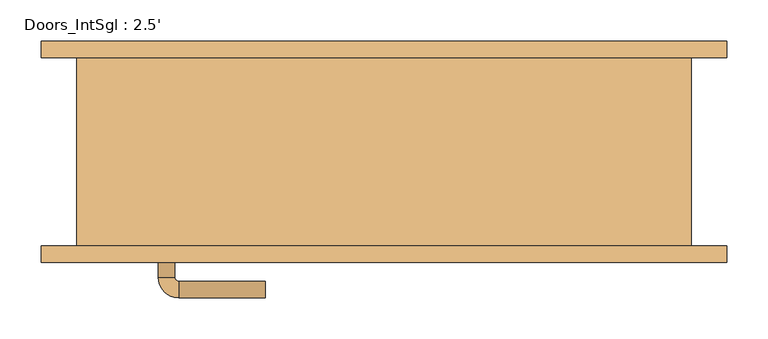
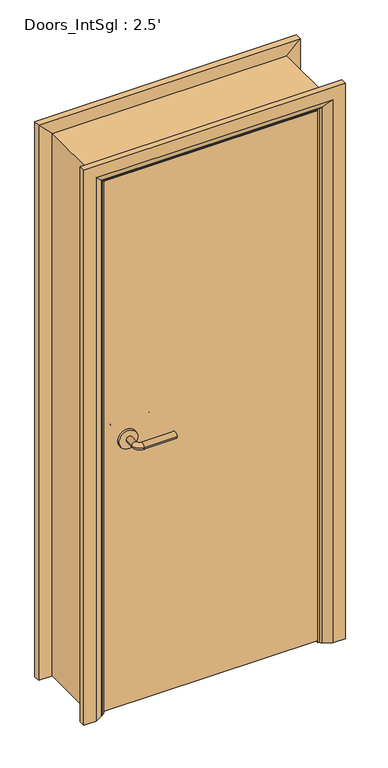
"""IFC4 building model written with IfcOpenShell, lengths in millimetres: door geometry, Doors_IntSgl : 2.5'."""

from ifc_helpers import new_model, si_unit, point, frame, frame_2d, origin, place, context, project, spatial, polyline, circle_curve, ellipse_curve, trimmed, segment, composite_curve, outline, extrude, faceted_brep, source, transform, mapped, element, save
from ifc_brep_helpers import plane_surface, cylinder_surface, revolved_surface, advanced_brep


def doors_intsgl_2_5_5ac032e7(model_context):
    return source(origin(), model_context, "Body", "SolidModel", [
        advanced_brep(
        [(-274.0, -68.3, 900.0), (-254.0, -68.3, 900.0), (-274.0, -38.3, 900.0), (-254.0, -38.3, 900.0), (-249.0, -33.3, 900.0), (-249.0, -13.3, 900.0), (-144.0, -13.3, 900.0), (-144.0, -33.3, 900.0)],
        [
            (0, 1, circle_curve(frame((-264.0, -68.3, 900.0), z_axis=(0.0, -1.0, 0.0), x_axis=(1.0, 0.0, 0.0)), 10.0)),
            (1, 0, circle_curve(frame((-264.0, -68.3, 900.0), z_axis=(0.0, -1.0, 0.0), x_axis=(1.0, 0.0, 0.0)), 10.0)),
            (0, 2),
            (2, 3, circle_curve(frame((-264.0, -38.3, 900.0), z_axis=(0.0, -1.0, 0.0), x_axis=(1.0, 0.0, 0.0)), 10.0)),
            (3, 1),
            (3, 2, circle_curve(frame((-264.0, -38.3, 900.0), z_axis=(0.0, -1.0, 0.0), x_axis=(1.0, 0.0, 0.0)), 10.0)),
            (4, 3, circle_curve(frame((-249.0, -38.3, 900.0), z_axis=(0.0, 0.0, 1.0), x_axis=(-1.0, 0.0, 0.0)), 5.0)),
            (2, 5, circle_curve(frame((-249.0, -38.3, 900.0), z_axis=(0.0, 0.0, -1.0), x_axis=(-1.0, 0.0, 0.0)), 25.0)),
            (5, 4, circle_curve(frame((-249.0, -23.3, 900.0), z_axis=(-1.0, 0.0, 0.0), x_axis=(0.0, -1.0, 0.0)), 10.0)),
            (4, 5, circle_curve(frame((-249.0, -23.3, 900.0), z_axis=(-1.0, 0.0, 0.0), x_axis=(0.0, -1.0, 0.0)), 10.0)),
            (6, 7, circle_curve(frame((-144.0, -23.3, 900.0), z_axis=(1.0, 0.0, 0.0), x_axis=(0.0, -1.0, 0.0)), 10.0)),
            (7, 6, circle_curve(frame((-144.0, -23.3, 900.0), z_axis=(1.0, 0.0, 0.0), x_axis=(0.0, -1.0, 0.0)), 10.0)),
            (5, 6),
            (7, 4),
        ],
        [
            plane_surface(frame((-264.0, -68.3, 900.0), z_axis=(0.0, -1.0, 0.0), x_axis=(0.0, 0.0, 1.0))),
            cylinder_surface(frame((-264.0, -68.3, 900.0), z_axis=(0.0, -1.0, 0.0), x_axis=(1.0, 0.0, 0.0)), 10.0),
            revolved_surface(trimmed(ellipse_curve(frame((-264.0, -38.3, 900.0), z_axis=(0.0, -1.0, 0.0), x_axis=(1.0, 0.0, 0.0)), 10.0, 10.0), [point((-274.0, -38.3, 900.0))], [point((-254.0, -38.3, 900.0))], True, "CARTESIAN"), (-249.0, -38.3, 900.0), (0.0, 0.0, -1.0)),
            revolved_surface(trimmed(ellipse_curve(frame((-264.0, -38.3, 900.0), z_axis=(0.0, -1.0, 0.0), x_axis=(1.0, 0.0, 0.0)), 10.0, 10.0), [point((-254.0, -38.3, 900.0))], [point((-274.0, -38.3, 900.0))], True, "CARTESIAN"), (-249.0, -38.3, 900.0), (0.0, 0.0, -1.0)),
            plane_surface(frame((-144.0, -23.3, 900.0), z_axis=(1.0, 0.0, 0.0), x_axis=(0.0, 0.0, 1.0))),
            cylinder_surface(frame((-249.0, -23.3, 900.0), z_axis=(-1.0, 0.0, 0.0), x_axis=(0.0, -1.0, 0.0)), 10.0),
        ],
        [
            (0, [[1, 2]]),
            (1, [[-1, 3, 4, 5]]),
            (1, [[-2, -5, 6, -3]]),
            (2, [[7, -4, 8, 9]]),
            (3, [[-8, -6, -7, 10]]),
            (4, [[11, 12]]),
            (5, [[-9, 13, -12, 14]]),
            (5, [[-10, -14, -11, -13]]),
        ],
    ),
        extrude(outline(composite_curve([segment(trimmed(circle_curve(frame_2d((900.0, -266.5)), 30.0), [point((900.0, -296.5))], [point((900.0, -236.5))], False, "CARTESIAN"), True, "CONTINUOUS"), segment(trimmed(circle_curve(frame_2d((900.0, -266.5)), 30.0), [point((900.0, -236.5))], [point((900.0, -296.5))], False, "CARTESIAN"), True, "CONTINUOUS")], self_intersect=False)), frame((0.0, -76.3, 0.0), z_axis=(0.0, 1.0, 0.0), x_axis=(0.0, 0.0, 1.0)), (0.0, 0.0, 1.0), 8.0),
        advanced_brep(
        [(-274.0, -122.3, 900.0), (-254.0, -122.3, 900.0), (-254.0, -152.3, 900.0), (-274.0, -152.3, 900.0), (-249.0, -157.3, 900.0), (-249.0, -177.3, 900.0), (-144.0, -177.3, 900.0), (-144.0, -157.3, 900.0)],
        [
            (0, 1, circle_curve(frame((-264.0, -122.3, 900.0), z_axis=(0.0, 1.0, 0.0), x_axis=(1.0, 0.0, 0.0)), 10.0)),
            (1, 0, circle_curve(frame((-264.0, -122.3, 900.0), z_axis=(0.0, 1.0, 0.0), x_axis=(1.0, 0.0, 0.0)), 10.0)),
            (1, 2),
            (2, 3, circle_curve(frame((-264.0, -152.3, 900.0), z_axis=(0.0, 1.0, 0.0), x_axis=(1.0, 0.0, 0.0)), 10.0)),
            (3, 0),
            (3, 2, circle_curve(frame((-264.0, -152.3, 900.0), z_axis=(0.0, 1.0, 0.0), x_axis=(1.0, 0.0, 0.0)), 10.0)),
            (4, 5, circle_curve(frame((-249.0, -167.3, 900.0), z_axis=(-1.0, 0.0, 0.0), x_axis=(0.0, 1.0, 0.0)), 10.0)),
            (5, 3, circle_curve(frame((-249.0, -152.3, 900.0), z_axis=(0.0, 0.0, -1.0), x_axis=(-1.0, 0.0, 0.0)), 25.0)),
            (2, 4, circle_curve(frame((-249.0, -152.3, 900.0), z_axis=(0.0, 0.0, 1.0), x_axis=(-1.0, 0.0, 0.0)), 5.0)),
            (5, 4, circle_curve(frame((-249.0, -167.3, 900.0), z_axis=(-1.0, 0.0, 0.0), x_axis=(0.0, 1.0, 0.0)), 10.0)),
            (6, 7, circle_curve(frame((-144.0, -167.3, 900.0), z_axis=(1.0, 0.0, 0.0), x_axis=(0.0, 1.0, 0.0)), 10.0)),
            (7, 6, circle_curve(frame((-144.0, -167.3, 900.0), z_axis=(1.0, 0.0, 0.0), x_axis=(0.0, 1.0, 0.0)), 10.0)),
            (4, 7),
            (6, 5),
        ],
        [
            plane_surface(frame((-264.0, -122.3, 900.0), z_axis=(0.0, 1.0, 0.0), x_axis=(0.0, 0.0, 1.0))),
            cylinder_surface(frame((-264.0, -122.3, 900.0), z_axis=(0.0, 1.0, 0.0), x_axis=(1.0, 0.0, 0.0)), 10.0),
            revolved_surface(trimmed(ellipse_curve(frame((-264.0, -152.3, 900.0), z_axis=(0.0, -1.0, 0.0), x_axis=(1.0, 0.0, 0.0)), 10.0, 10.0), [point((-274.0, -152.3, 900.0))], [point((-254.0, -152.3, 900.0))], True, "CARTESIAN"), (-249.0, -152.3, 900.0), (0.0, 0.0, -1.0)),
            revolved_surface(trimmed(ellipse_curve(frame((-264.0, -152.3, 900.0), z_axis=(0.0, -1.0, 0.0), x_axis=(1.0, 0.0, 0.0)), 10.0, 10.0), [point((-254.0, -152.3, 900.0))], [point((-274.0, -152.3, 900.0))], True, "CARTESIAN"), (-249.0, -152.3, 900.0), (0.0, 0.0, -1.0)),
            plane_surface(frame((-144.0, -167.3, 900.0), z_axis=(1.0, 0.0, 0.0), x_axis=(0.0, 0.0, 1.0))),
            cylinder_surface(frame((-249.0, -167.3, 900.0), z_axis=(-1.0, 0.0, 0.0), x_axis=(0.0, 1.0, 0.0)), 10.0),
        ],
        [
            (0, [[1, 2]]),
            (1, [[3, 4, 5, -2]]),
            (1, [[-5, 6, -3, -1]]),
            (2, [[7, 8, -4, 9]]),
            (3, [[10, -9, -6, -8]]),
            (4, [[11, 12]]),
            (5, [[13, -11, 14, -7]]),
            (5, [[-14, -12, -13, -10]]),
        ],
    ),
        extrude(outline(composite_curve([segment(trimmed(circle_curve(frame_2d((900.0, -266.5)), 30.0), [point((900.0, -296.5))], [point((900.0, -236.5))], False, "CARTESIAN"), True, "CONTINUOUS"), segment(trimmed(circle_curve(frame_2d((900.0, -266.5)), 30.0), [point((900.0, -236.5))], [point((900.0, -296.5))], False, "CARTESIAN"), True, "CONTINUOUS")], self_intersect=False)), frame((0.0, -122.3, 0.0), z_axis=(0.0, 1.0, 0.0), x_axis=(0.0, 0.0, 1.0)), (0.0, 0.0, 1.0), 8.0),
        extrude(outline(polyline([(339.0, -76.3), (339.0, -114.3), (-339.0, -114.3), (-339.0, -76.3), (339.0, -76.3)])), frame((0.0, 0.0, 8.0), z_axis=(0.0, 0.0, 1.0), x_axis=(1.0, 0.0, 0.0)), (0.0, 0.0, 1.0), 1778.8),
        advanced_brep(
        [(416.0, -134.3, 0.0), (376.0, -134.3, 0.0), (350.0, -120.3, 0.0), (346.0, -114.3, 0.0), (416.0, -114.3, 0.0), (416.0, -114.3, 1863.8), (416.0, -134.3, 1863.8), (346.0, -114.3, 1793.8), (-346.0, -114.3, 1793.8), (-346.0, -114.3, 0.0), (-416.0, -114.3, 0.0), (-416.0, -114.3, 1863.8), (350.0, -120.3, 1797.8), (376.0, -134.3, 1823.8), (-416.0, -134.3, 1863.8), (-416.0, -134.3, 0.0), (-376.0, -134.3, 0.0), (-376.0, -134.3, 1823.8), (-350.0, -120.3, 0.0), (-350.0, -120.3, 1797.8)],
        [
            (0, 1),
            (1, 2),
            (2, 3, circle_curve(frame((354.0, -113.3, 0.0), z_axis=(0.0, 0.0, -1.0), x_axis=(1.0, 0.0, 0.0)), 8.0622577)),
            (3, 4),
            (4, 0),
            (4, 5),
            (5, 6),
            (6, 0),
            (3, 7),
            (7, 8),
            (8, 9),
            (9, 10),
            (10, 11),
            (11, 5),
            (2, 12),
            (12, 7, ellipse_curve(frame((354.0, -113.3, 1801.8), z_axis=(0.7071067811865475, 0.0, -0.7071067811865475), x_axis=(-0.7071067811865474, 0.0, -0.7071067811865476)), 11.4017543, 8.0622577)),
            (1, 13),
            (13, 12),
            (6, 14),
            (14, 15),
            (15, 16),
            (16, 17),
            (17, 13),
            (10, 15),
            (14, 11),
            (9, 18, circle_curve(frame((-354.0, -113.3, 0.0), z_axis=(0.0, 0.0, -1.0), x_axis=(-1.0, 0.0, 0.0)), 8.0622577)),
            (18, 16),
            (19, 18),
            (8, 19, ellipse_curve(frame((-354.0, -113.3, 1801.8), z_axis=(-0.7071067811865475, 0.0, -0.7071067811865475), x_axis=(-0.7071067811865474, 0.0, 0.7071067811865476)), 11.4017543, 8.0622577)),
            (19, 17),
            (12, 19),
        ],
        [
            plane_surface(frame((346.0, -114.3, 0.0), z_axis=(0.0, 0.0, -1.0), x_axis=(0.0, 1.0, 0.0))),
            plane_surface(frame((416.0, -134.3, 0.0), z_axis=(1.0, 0.0, 0.0), x_axis=(0.0, 0.0, 1.0))),
            plane_surface(frame((416.0, -114.3, 0.0), z_axis=(0.0, 1.0, 0.0), x_axis=(0.0, 0.0, 1.0))),
            cylinder_surface(frame((354.0, -113.3, 0.0), z_axis=(0.0, 0.0, -1.0), x_axis=(1.0, 0.0, 0.0)), 8.0622577),
            plane_surface(frame((350.0, -120.3, 0.0), z_axis=(-0.4740998230350126, -0.880471099922178, 0.0), x_axis=(0.0, 0.0, 1.0))),
            plane_surface(frame((376.0, -134.3, 0.0), z_axis=(0.0, -1.0, 0.0), x_axis=(0.0, 0.0, 1.0))),
            plane_surface(frame((-416.0, -134.3, 1863.8), z_axis=(-1.0, 0.0, 0.0), x_axis=(0.0, 0.0, -1.0))),
            plane_surface(frame((-346.0, -114.3, 0.0), z_axis=(0.0, 0.0, -1.0), x_axis=(0.0, 1.0, 0.0))),
            cylinder_surface(frame((-354.0, -113.3, 1793.8), z_axis=(0.0, 0.0, 1.0), x_axis=(-1.0, 0.0, 0.0)), 8.0622577),
            plane_surface(frame((-350.0, -120.3, 1797.8), z_axis=(0.47409982303501824, -0.8804710999221749, 0.0), x_axis=(0.0, 0.0, -1.0))),
            plane_surface(frame((416.0, -134.3, 1863.8), z_axis=(0.0, 0.0, 1.0), x_axis=(-1.0, 0.0, 0.0))),
            cylinder_surface(frame((346.0, -113.3, 1801.8), z_axis=(1.0, 0.0, 0.0), x_axis=(0.0, 0.0, 1.0)), 8.0622577),
            plane_surface(frame((350.0, -120.3, 1797.8), z_axis=(0.0, -0.8804710999221764, -0.4740998230350154), x_axis=(-1.0, 0.0, 0.0))),
        ],
        [
            (0, [[1, 2, 3, 4, 5]]),
            (1, [[6, 7, 8, -5]]),
            (2, [[9, 10, 11, 12, 13, 14, -6, -4]]),
            (3, [[15, 16, -9, -3]]),
            (4, [[17, 18, -15, -2]]),
            (5, [[-8, 19, 20, 21, 22, 23, -17, -1]]),
            (6, [[-13, 24, -20, 25]]),
            (7, [[-24, -12, 26, 27, -21]]),
            (8, [[28, -26, -11, 29]]),
            (9, [[-22, -27, -28, 30]]),
            (10, [[-14, -25, -19, -7]]),
            (11, [[31, -29, -10, -16]]),
            (12, [[-23, -30, -31, -18]]),
        ],
    ),
        extrude(outline(polyline([(0.0, -322.0), (1769.8, -322.0), (1769.8, 322.0), (0.0, 322.0), (0.0, 341.0), (1788.8, 341.0), (1788.8, -341.0), (0.0, -341.0), (0.0, -322.0)])), frame((0.0, -74.3, 0.0), z_axis=(0.0, 1.0, 0.0), x_axis=(0.0, 0.0, 1.0)), (0.0, 0.0, 1.0), 32.0),
        advanced_brep(
        [(-416.0, 134.3, 0.0), (-376.0, 134.3, 0.0), (-350.0, 120.3, 0.0), (-346.0, 114.3, 0.0), (-416.0, 114.3, 0.0), (-416.0, 114.3, 1863.8), (-416.0, 134.3, 1863.8), (-346.0, 114.3, 1793.8), (-350.0, 120.3, 1797.8), (-376.0, 134.3, 1823.8), (416.0, 134.3, 0.0), (416.0, 114.3, 0.0), (346.0, 114.3, 0.0), (350.0, 120.3, 0.0), (376.0, 134.3, 0.0), (416.0, 134.3, 1863.8), (376.0, 134.3, 1823.8), (350.0, 120.3, 1797.8), (346.0, 114.3, 1793.8), (416.0, 114.3, 1863.8)],
        [
            (0, 1),
            (1, 2),
            (2, 3, circle_curve(frame((-354.0, 113.3, 0.0), z_axis=(0.0, 0.0, -1.0), x_axis=(-1.0, 0.0, 0.0)), 8.0622577)),
            (3, 4),
            (4, 0),
            (4, 5),
            (5, 6),
            (6, 0),
            (3, 7),
            (7, 5),
            (2, 8),
            (8, 7, ellipse_curve(frame((-354.0, 113.3, 1801.8), z_axis=(-0.7071067811865475, 0.0, -0.7071067811865475), x_axis=(0.7071067811865474, 0.0, -0.7071067811865476)), 11.4017543, 8.0622577)),
            (1, 9),
            (9, 8),
            (6, 9),
            (10, 11),
            (11, 12),
            (12, 13, circle_curve(frame((354.0, 113.3, 0.0), z_axis=(0.0, 0.0, -1.0), x_axis=(1.0, 0.0, 0.0)), 8.0622577)),
            (13, 14),
            (14, 10),
            (15, 10),
            (14, 16),
            (16, 15),
            (13, 17),
            (17, 16),
            (12, 18),
            (18, 17, ellipse_curve(frame((354.0, 113.3, 1801.8), z_axis=(0.7071067811865475, 0.0, -0.7071067811865475), x_axis=(0.7071067811865474, 0.0, 0.7071067811865476)), 11.4017543, 8.0622577)),
            (11, 19),
            (19, 18),
            (15, 19),
            (5, 19),
            (15, 6),
            (7, 18),
            (8, 17),
            (9, 16),
        ],
        [
            plane_surface(frame((-346.0, 187.1010989, 0.0), z_axis=(0.0, 0.0, -1.0), x_axis=(1.0, 0.0, 0.0))),
            plane_surface(frame((-416.0, 134.3, 0.0), z_axis=(-1.0, 0.0, 0.0), x_axis=(0.0, 0.0, 1.0))),
            plane_surface(frame((-416.0, 114.3, 0.0), z_axis=(0.0, -1.0, 0.0), x_axis=(0.0, 0.0, 1.0))),
            cylinder_surface(frame((-354.0, 113.3, 0.0), z_axis=(0.0, 0.0, -1.0), x_axis=(-1.0, 0.0, 0.0)), 8.0622577),
            plane_surface(frame((-350.0, 120.3, 0.0), z_axis=(0.4740998230350183, 0.8804710999221749, 0.0), x_axis=(0.0, 0.0, 1.0))),
            plane_surface(frame((-376.0, 134.3, 0.0), z_axis=(0.0, 1.0, 0.0), x_axis=(0.0, 0.0, 1.0))),
            plane_surface(frame((346.0, 187.1010989, 0.0), z_axis=(0.0, 0.0, -1.0), x_axis=(-1.0, 0.0, 0.0))),
            plane_surface(frame((376.0, 134.3, 1823.8), z_axis=(0.0, 1.0, 0.0), x_axis=(0.0, 0.0, -1.0))),
            plane_surface(frame((350.0, 120.3, 1797.8), z_axis=(-0.4740998230350183, 0.8804710999221749, 0.0), x_axis=(0.0, 0.0, -1.0))),
            cylinder_surface(frame((354.0, 113.3, 1793.8), z_axis=(0.0, 0.0, 1.0), x_axis=(1.0, 0.0, 0.0)), 8.0622577),
            plane_surface(frame((416.0, 114.3, 1863.8), z_axis=(0.0, -1.0, 0.0), x_axis=(0.0, 0.0, -1.0))),
            plane_surface(frame((416.0, 134.3, 1863.8), z_axis=(1.0, 0.0, 0.0), x_axis=(0.0, 0.0, -1.0))),
            plane_surface(frame((-416.0, 134.3, 1863.8), z_axis=(0.0, 0.0, 1.0), x_axis=(1.0, 0.0, 0.0))),
            plane_surface(frame((-416.0, 114.3, 1863.8), z_axis=(0.0, -1.0, 0.0), x_axis=(1.0, 0.0, 0.0))),
            cylinder_surface(frame((-346.0, 113.3, 1801.8), z_axis=(-1.0, 0.0, 0.0), x_axis=(0.0, 0.0, 1.0)), 8.0622577),
            plane_surface(frame((-350.0, 120.3, 1797.8), z_axis=(0.0, 0.8804710999221749, -0.4740998230350183), x_axis=(1.0, 0.0, 0.0))),
            plane_surface(frame((-376.0, 134.3, 1823.8), z_axis=(0.0, 1.0, 0.0), x_axis=(1.0, 0.0, 0.0))),
        ],
        [
            (0, [[1, 2, 3, 4, 5]]),
            (1, [[6, 7, 8, -5]]),
            (2, [[9, 10, -6, -4]]),
            (3, [[11, 12, -9, -3]]),
            (4, [[13, 14, -11, -2]]),
            (5, [[-8, 15, -13, -1]]),
            (6, [[16, 17, 18, 19, 20]]),
            (7, [[21, -20, 22, 23]]),
            (8, [[-22, -19, 24, 25]]),
            (9, [[-24, -18, 26, 27]]),
            (10, [[-26, -17, 28, 29]]),
            (11, [[-28, -16, -21, 30]]),
            (12, [[31, -30, 32, -7]]),
            (13, [[33, -29, -31, -10]]),
            (14, [[34, -27, -33, -12]]),
            (15, [[35, -25, -34, -14]]),
            (16, [[-32, -23, -35, -15]]),
        ],
    ),
        faceted_brep([(-341.0, -114.3, 0.0), (-373.0, -114.3, 0.0), (-373.0, 114.3, 0.0), (-341.0, 114.3, 0.0), (-341.0, 114.3, 1788.8), (-341.0, -114.3, 1788.8), (-373.0, 114.3, 1820.8), (-373.0, -114.3, 1820.8), (341.0, -114.3, 0.0), (341.0, 114.3, 0.0), (373.0, 114.3, 0.0), (373.0, -114.3, 0.0), (341.0, -114.3, 1788.8), (373.0, -114.3, 1820.8), (373.0, 114.3, 1820.8), (341.0, 114.3, 1788.8)], [[[0, 1, 2, 3]], [[3, 4, 5, 0]], [[2, 6, 4, 3]], [[1, 7, 6, 2]], [[0, 5, 7, 1]], [[8, 9, 10, 11]], [[12, 8, 11, 13]], [[13, 11, 10, 14]], [[14, 10, 9, 15]], [[15, 9, 8, 12]], [[4, 15, 12, 5]], [[6, 14, 15, 4]], [[7, 13, 14, 6]], [[5, 12, 13, 7]]]),
    ])


if __name__ == "__main__":
    model = new_model("IFC4")
    model_context = context("Model", 3, world=origin())
    ifc_project = project(units=[si_unit("LENGTHUNIT", "METRE", prefix="MILLI")], contexts=[model_context])
    site = spatial("IfcSite", under=ifc_project)
    building = spatial("IfcBuilding", under=site)
    placement = place(None, origin())
    doors_intsgl_2_5_shape = doors_intsgl_2_5_5ac032e7(model_context)
    element("IfcDoor", 1, ObjectType="Doors_IntSgl : 2.5'", at=placement, inside=building, context=model_context, shape_type="MappedRepresentation", body=[
        mapped(doors_intsgl_2_5_shape, transform((0.0, 0.0, 0.0), x_axis=(1.0, 0.0, 0.0), y_axis=(0.0, 1.0, 0.0), z_axis=(0.0, 0.0, 1.0))),
    ])
    save(model, "model.ifc")

# Revit data of these elements
# Type "Doors_IntSgl : 2.5'"
#   Type Mark = "49"
#   Type Comments = "Internal Single"
#   Operation = "SingleSwingRight"
#   Manufacturer = "Revit"
#   Keynote = "L20"
#   Description = "Internal Single Door"
#   Analytic Construction = "Metal"
#   UnderCut = 0' - 0.31496"
#   Tolerance = 0' - 0.07874"
#   Thickness = 0' - 1.49606"
#   Thermal Resistance (R) = 0.270117 (m²·K)/W
#   Structural Tolerance = 0' - 0.31496"
#   StopDepth = 0' - 1.25984"
#   Stop Thickness = 0' - 0.74803"
#   Rough Width = 2' - 6"
#   Rough Height = 6' - 0"
#   Height to Top Lock Rail = 3' - 3.37008"
#   Heat Transfer Coefficient (U) = 3.7021 W/(m²·K)
#   Handle Z Distance = 2' - 11.43307"
#   Handle X Distance = 0' - 2.95276"
#   Frame Thickness = 0' - 1.25984"
#   Door Panel Width = 2' - 2.69291"
#   Door Panel Thickness = 0' - 1.49606"
#   Door Panel Offset = 0' - 0"
#   Height = 6' - 0"
#   Width = 2' - 6"
#   Door Panel Height = 5' - 10.0315"
#   Architrave Setback = 0' - 0.19685"
#   Vis - Ironmongery = yes
#   Material Ironmongery = Door - Handle
#   Material Frame = Door - Frame/Mullion (1)
#   Material Door = Door - Panel
#   Material Architrave = Door - Architrave
#   Visual Light Transmittance = 0
#   Solar Heat Gain Coefficient = 0
#   Function = (empty or 0)
#   Wall Closure = (empty or 0)
# Element 1 (IfcDoor, "Doors_IntSgl : 2.5'")
#   Materials on its faces: "Door - Architrave", "Door - Handle", "Door - Frame/Mullion (1)", "Door - Panel"
# Materials
#   "Door - Handle": colour RGB 0 0 0, transparency 0, Keynote = "P21", Cost = 0
#   "Door - Frame/Mullion (1)": class "Wood", colour RGB 212 179 113, transparency 0, Keynote = "L20", Cost = 0
#   "Door - Panel": class "Wood", colour RGB 210 159 95, transparency 0, Keynote = "L20", Cost = 0
#   "Door - Architrave": class "Wood", colour RGB 154 90 5, transparency 0, Keynote = "P20", Cost = 0
